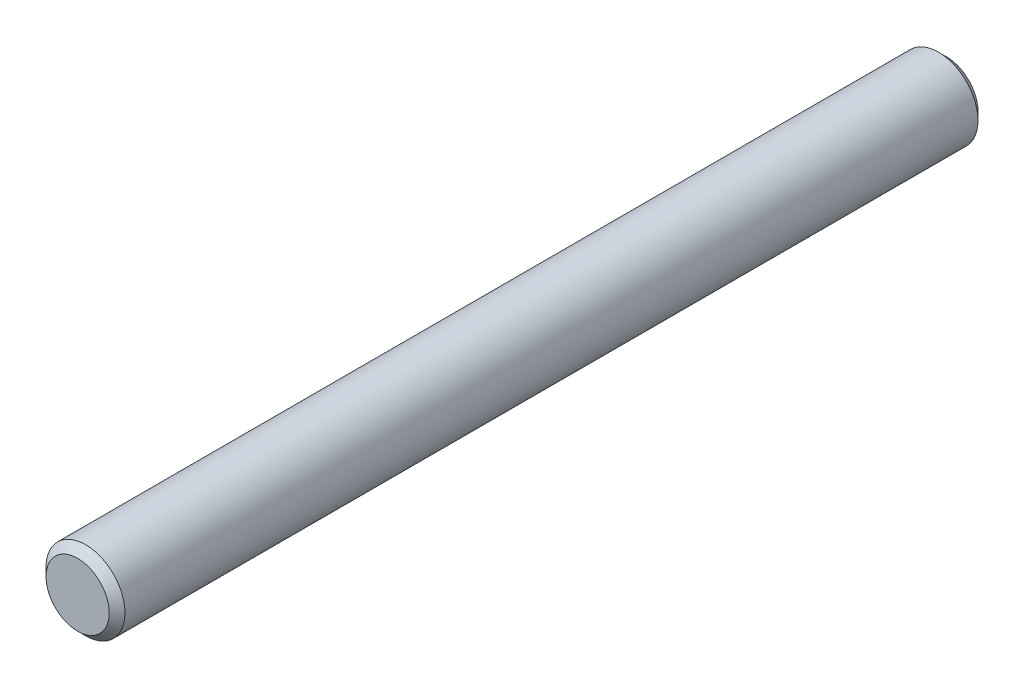
SolidWorks part; units mm, degrees
material "Plain Carbon Steel"
ref_plane "Front Plane" through (0, 0, 0) normal (0, 0, 1) x (1, 0, 0)
ref_plane "Top Plane" through (0, 0, 0) normal (0, 1, 0) x (1, 0, 0)
ref_plane "Right Plane" through (0, 0, 0) normal (1, 0, 0) x (0, 0, -1)
sketch "Pin Profile Ø5" plane through (0, 0, 0) normal (0, 0, 1) x (1, 0, 0)
  circle A0 centre (0, 0) radius 2.5
  dimension "D1" = 5
extrude "Pin Body Ø5x55" add sketch "Pin Profile Ø5" along normal mid plane 55
chamfer "End Chamfers 0.5x45°" distance 0.5 angle 45 2 edges at (2.5, 0, -27.5) (2.5, 0, 27.5)
